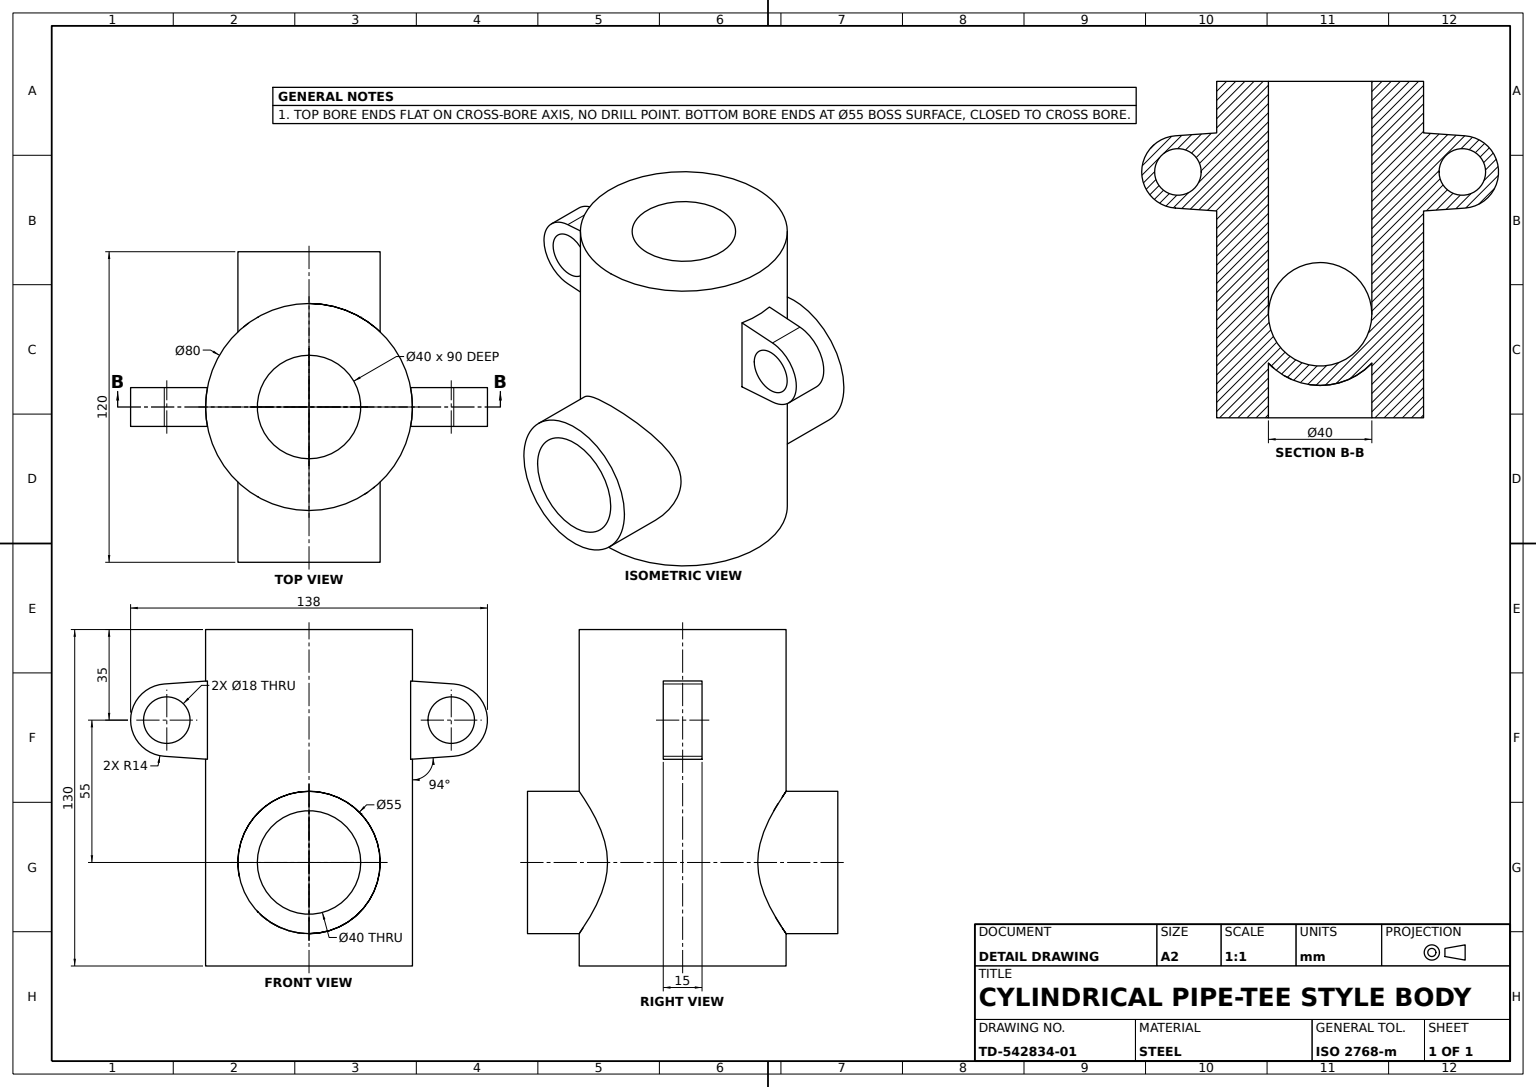
SolidWorks part; units mm, degrees
material "Plain Carbon Steel"
ref_plane "Front Plane" through (0, 0, 0) normal (0, 0, 1) x (1, 0, 0)
ref_plane "Top Plane" through (0, 0, 0) normal (0, 1, 0) x (1, 0, 0)
ref_plane "Right Plane" through (0, 0, 0) normal (1, 0, 0) x (0, 0, -1)
sketch "Main Body Sketch" plane through (0, 0, 0) normal (0, 1, 0) x (1, 0, 0)
  circle A0 centre (0, 0) radius 40
  circle A1 centre (0, 0) radius 20
  dimension "D1" = 80
  dimension "D2" = 40
extrude "Main Body" add sketch "Main Body Sketch" along normal blind 130
sketch "Cross Boss Sketch" plane through (0, 0, 0) normal (0, 0, 1) x (1, 0, 0)
  line L0 (-40, 0) -> (40, 0) construction
  circle A0 centre (0, 40) radius 27.5
  circle A1 centre (0, 40) radius 20
  dimension "D1" = 55
  dimension "D2" = 40
  dimension "D3" = 40
extrude "Cross Boss" add sketch "Cross Boss Sketch" along normal mid plane 120
sketch "Mounting Lugs Sketch" plane through (0, 0, 0) normal (0, 0, 1) x (1, 0, 0)
  line L2 (0, 0) -> (0, 179.0324)
  line L3 (-40, 0) -> (40, 0) construction
  line L4 (-55.9766, 108.9659) -> (-23.1647, 111.2603)
  line L5 (-55.9766, 81.0341) -> (-19.9242, 78.5131)
  line L6 (55.9766, 108.9659) -> (23.2158, 111.2568)
  line L7 (55.9766, 81.0341) -> (24.8387, 78.8567)
  line L8 (-23.1647, 111.2603) -> (23.2158, 111.2568)
  line L9 (24.8387, 78.8567) -> (-19.9242, 78.5131)
  circle A0 centre (-55, 95) radius 9
  circle A1 centre (55, 95) radius 9
  arc A2 (-55.9766, 108.9659) -> (-55.9766, 81.0341) centre (-55, 95) ccw
  arc A3 (55.9766, 81.0341) -> (55.9766, 108.9659) centre (55, 95) ccw
  dimension "D4" = 18
  dimension "D5" = 18
  dimension "D6" = 28
  dimension "D7" = 28
  dimension "D2" = 55
  dimension "D3" = 55
  dimension "D8" = 8
  dimension "D9" = 95
  dimension "D10" = 8
  dimension "D11" = 86
  dimension "D12" = 86
  dimension "D13" = 32.8921
  dimension "D14" = 36.1404
  dimension "D15" = 32.8408
  dimension "D16" = 31.2139
  dimension "D17" = 179.0324
extrude "Mounting Lugs" add sketch "Mounting Lugs Sketch" along normal mid plane 15 contours L4 A2 L5 L9 L2 L8 A0 | L7 A3 L6 L8 L2 L9 A1
sketch "Top Bore Sketch" plane through (0, 130, 0) normal (0, 1, 0) x (1, 0, 0)
  circle A0 centre (0, 0) radius 20
  dimension "D1" = 40
extrude "Top Bore" cut sketch "Top Bore Sketch" against normal blind 90
sketch "Cross Bore Sketch" plane through (0, 0, 60) normal (0, 0, 1) x (1, 0, 0)
  circle A0 centre (0, 40) radius 20
  dimension "D1" = 40
extrude "Cross Bore" cut sketch "Cross Bore Sketch" against normal blind 150
